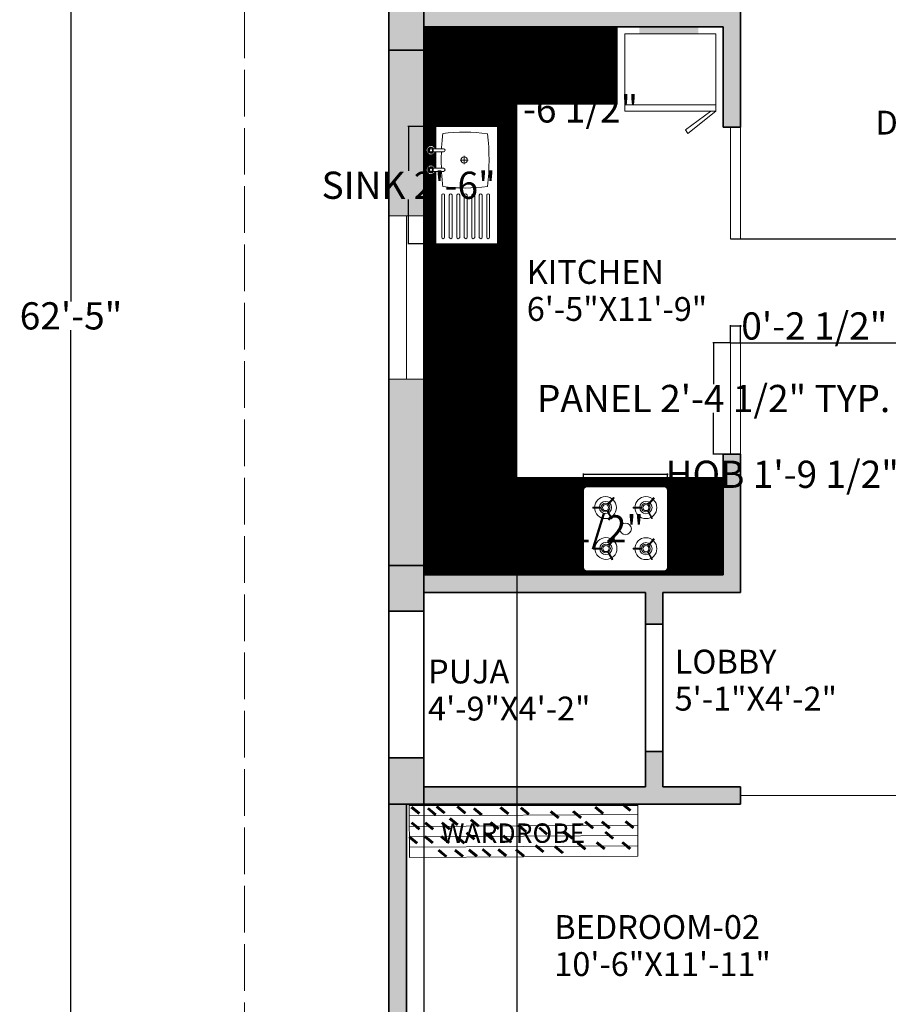
# Model space of a CAD drawing. Units: inches. Extents: x -17 to 892, y -721 to 172.
# Tile 2 of 11: x -12 to 212, y -462 to -209. Entities that reach past the tile are written whole.
import ezdxf

# ---------------------------------------------------------------- set-up
doc = ezdxf.new("R2010")
doc.units = ezdxf.units.IN
doc.header["$MEASUREMENT"] = 0
doc.linetypes.add('ACAD_ISO02W100', pattern=[15, 12, -3])
doc.layers.get('0').update_dxf_attribs({"color": 14})
for name, color, linetype, lineweight in [('A-ANNO-DIMS', 2, 'Continuous', 18), ('A-ANNO-TEXT', 7, 'Continuous', 18), ('A-AREA-IDEN', 7, 'Continuous', 18), ('A-COLS', 252, 'Continuous', 35), ('A-EQPM', 8, 'Continuous', 18), ('A-FLOR-CASE', 252, 'Continuous', 18), ('A-FLOR-FIXT', 8, 'Continuous', 18), ('A-FURN-PATT', 252, 'Continuous', 9), ('A-WALL-PATT', 14, 'Continuous', 13), ('C-PROP', 8, 'ACAD_ISO02W100', 18), ('doors', 4, 'Continuous', 18), ('furniture', 252, 'Continuous', 18), ('walls', 252, 'Continuous', 35), ('windows', 161, 'Continuous', 18)]:
    doc.layers.add(name, color=color, linetype=linetype, lineweight=lineweight)
doc.layers.add('A-COLS-PATT', color=254, linetype='Continuous', lineweight=13, true_color=0xd7ebd2)
doc.layers.add('A-FLOR-CASE-PATT', color=51, linetype='Continuous', lineweight=13, true_color=0xf8f6b0)
doc.styles.get("Standard").update_dxf_attribs({"font": 'arial.ttf'})
doc.dimstyles.get("Standard").update_dxf_attribs({"dimtxt": 7, "dimasz": 0.18, "dimexe": 0.18, "dimexo": 0.0625, "dimgap": 0.09, "dimtad": 0, "dimtih": 1, "dimtoh": 1, "dimzin": 0, "dimdsep": 46, "dimlunit": 3, "dimtxsty": 'Standard', "dimcen": 0.09, "dimadec": 0, "dimazin": 0, "dimtfac": 1, "dimtofl": 0, "dimtmove": 0, "dimatfit": 3, "dimfxl": 1, "dimtolj": 1, "dimtzin": 0, "dimarcsym": 0})

# ---------------------------------------------------------------- blocks, each defined once
blk = doc.blocks.new('A$C799204C7')
for p, q in [((0, 34.2), (17.99, 34.2)), ((0, 0), (0, 34.2)), ((2.32, 20.01), (2.32, 32.27)), ((3.13, 20.01), (3.13, 32.27)), ((4.48, 20.01), (4.48, 32.27)), ((5.29, 20.01), (5.29, 32.27)), ((6.64, 20.01), (6.64, 32.27)), ((7.45, 20.01), (7.45, 32.27)), ((8.85, 20.01), (8.85, 32.27)), ((9.66, 20.01), (9.66, 32.27)), ((11.01, 20.01), (11.01, 32.27)), ((11.82, 20.01), (11.82, 32.27)), ((13.22, 20.01), (13.22, 32.27)), ((14.03, 20.01), (14.03, 32.27)), ((15.42, 20.01), (15.42, 32.27)), ((16.24, 20.01), (16.24, 32.27)), ((17.99, 13.08), (17.99, 34.2)), ((18.59, 13.08), (15.71, 13.08)), ((15.71, 12.17), (18.59, 12.17)), ((17.99, 7.36), (17.99, 12.17)), ((8.52, 9.77), (10.9, 9.77)), ((9.73, 11), (9.73, 8.54)), ((18.59, 7.36), (15.71, 7.36)), ((15.71, 6.45), (18.59, 6.45)), ((17.99, 0), (17.99, 6.45)), ((0, 0), (17.99, 0))]:
    blk.add_line(p, q)
for centre, radius in [((19.38, 12.62), 0.684), ((19.38, 12.62), 0.456), ((9.7, 9.77), 0.916), ((19.38, 6.91), 0.684), ((19.38, 6.91), 0.456)]:
    blk.add_circle(centre, radius)
for centre, radius, start, end in [((2.72, 32.27), 0.407, 0, 180), ((4.88, 32.27), 0.407, 0, 180), ((7.05, 32.27), 0.407, 0, 180), ((9.25, 32.27), 0.407, 0, 180), ((11.42, 32.27), 0.407, 0, 180), ((13.62, 32.27), 0.407, 0, 180), ((15.83, 32.27), 0.407, 0, 180), ((2.72, 20.01), 0.407, 180, 0), ((67.33, 9.77), 64.88, 173.1952, 186.8048), ((9.53, -30.19), 48.1, 82.3437, 97.8966), ((4.88, 20.01), 0.407, 180, 0), ((7.05, 20.01), 0.407, 180, 0), ((9.25, 20.01), 0.407, 180, 0), ((11.42, 20.01), 0.407, 180, 0), ((13.62, 20.01), 0.407, 180, 0), ((15.83, 20.01), 0.407, 180, 0), ((-48.51, 9.77), 64.88, 2.9208, 6.8048), ((15.71, 12.62), 0.456, 90, 270), ((-48.51, 9.77), 64.88, 357.8723, 2.115), ((19.38, 12.62), 1.37, 199.6514, 160.3603), ((19.38, 12.62), 0.911, 210.3431, 149.7554), ((15.71, 6.91), 0.456, 90, 270), ((-48.51, 9.77), 64.88, 353.1952, 357.0665), ((19.38, 6.91), 1.37, 199.6514, 160.3603), ((19.38, 6.91), 0.911, 210.3431, 149.7554), ((9.53, 49.73), 48.1, 262.1034, 277.6563)]:
    blk.add_arc(centre, radius, start, end)
blk = doc.blocks.new('sink')
at = {"layer": 'furniture'}
for p, q in [((8718164203.894819, -1433730582.369047), (8718164201.504578, -1433730582.369047)), ((8718164202.684322, -1433730581.131674), (8718164202.684322, -1433730583.598095)), ((8718164196.150837, -1433730592.638258), (8718164196.150837, -1433730604.938997)), ((8718164196.967728, -1433730592.638258), (8718164196.967728, -1433730604.938997)), ((8718164198.365185, -1433730592.638258), (8718164198.365185, -1433730604.938997)), ((8718164199.182076, -1433730592.638258), (8718164199.182076, -1433730604.938997)), ((8718164200.579533, -1433730592.638258), (8718164200.579533, -1433730604.938997)), ((8718164201.396423, -1433730592.638258), (8718164201.396423, -1433730604.938997)), ((8718164202.748692, -1433730592.638258), (8718164202.748692, -1433730604.938997)), ((8718164203.565582, -1433730592.638258), (8718164203.565582, -1433730604.938997)), ((8718164204.963041, -1433730592.638258), (8718164204.963041, -1433730604.938997)), ((8718164205.779934, -1433730592.638258), (8718164205.779934, -1433730604.938997)), ((8718164207.1322, -1433730592.638258), (8718164207.1322, -1433730604.938997)), ((8718164207.949093, -1433730592.638258), (8718164207.949093, -1433730604.938997)), ((8718164209.301359, -1433730592.638258), (8718164209.301359, -1433730604.938997)), ((8718164210.118252, -1433730592.638258), (8718164210.118252, -1433730604.938997))]:
    blk.add_line(p, q, dxfattribs=at)
for centre, radius in [((8718164192.998869, -1433730579.495552), 0.685789), ((8718164192.998869, -1433730579.495552), 0.457192), ((8718164202.715019, -1433730582.369047), 0.919003), ((8718164192.998869, -1433730585.228166), 0.68579), ((8718164192.998869, -1433730585.228166), 0.68579), ((8718164192.998869, -1433730585.228166), 0.457192)]:
    blk.add_circle(centre, radius, dxfattribs=at)
for centre, radius, start, end in [((8718164196.559284, -1433730592.638258), 0.41045, 354.3355999, 185.6644001), ((8718164198.77363, -1433730592.638258), 0.41045, 354.3355999, 185.6644001), ((8718164200.98798, -1433730592.638258), 0.41045, 354.3355999, 185.6644001), ((8718164203.157139, -1433730592.638258), 0.41045, 354.3355999, 185.6644001), ((8718164205.371487, -1433730592.638258), 0.41045, 354.3355999, 185.6644001), ((8718164207.540646, -1433730592.640262), 0.41045, 354.3355999, 185.6644001), ((8718164209.709805, -1433730592.640262), 0.41045, 354.3355999, 185.6644001), ((8718164196.559284, -1433730604.938997), 0.408445, 180, 0), ((8718164198.77363, -1433730604.938997), 0.408445, 180, 0), ((8718164200.98798, -1433730604.938997), 0.408445, 180, 0), ((8718164203.157139, -1433730604.938997), 0.408445, 180, 0), ((8718164205.371487, -1433730604.938997), 0.408445, 180, 0), ((8718164207.540646, -1433730604.938997), 0.408445, 180, 0), ((8718164209.709805, -1433730604.938997), 0.408445, 180, 0)]:
    blk.add_arc(centre, radius, start, end, dxfattribs=at)
at = {"layer": 'furniture', "xscale": 1.0032, "yscale": 1.0032, "zscale": 1.0032, "rotation": 180}
blk.add_blockref('A$C799204C7', (8718164212.441259, -1433730572.566334), dxfattribs=at)
blk = doc.blocks.new('washbasin')
at = {"layer": 'furniture'}
blk.add_blockref('sink', (-8718164214.119328, 1433730589.721069), dxfattribs=at)
blk = doc.blocks.new('4bstove')
at = {"layer": 'furniture'}
for p, q in [((1452.73, 1446.21), (1452.73, 1448.61)), ((1452.98, 1446.22), (1452.98, 1448.61)), ((1464.44, 1446.34), (1464.44, 1448.73)), ((1464.69, 1446.34), (1464.69, 1448.73)), ((1451.74, 1444.45), (1449.67, 1443.25)), ((1451.87, 1444.23), (1449.79, 1443.04)), ((1453.91, 1444.27), (1455.74, 1442.73)), ((1463.45, 1444.58), (1461.38, 1443.38)), ((1463.57, 1444.36), (1461.5, 1443.17)), ((1465.46, 1444.21), (1467.29, 1442.67)), ((1465.62, 1444.4), (1467.45, 1442.86)), ((1453.75, 1444.08), (1455.58, 1442.54)), ((1452.69, 1434.81), (1452.69, 1437.2)), ((1452.94, 1434.81), (1452.94, 1437.2)), ((1464.44, 1434.81), (1464.44, 1437.2)), ((1464.69, 1434.81), (1464.69, 1437.2)), ((1451.7, 1433.04), (1449.63, 1431.85)), ((1463.45, 1433.04), (1461.38, 1431.85)), ((1451.82, 1432.83), (1449.75, 1431.63)), ((1453.71, 1432.67), (1455.54, 1431.13)), ((1453.87, 1432.86), (1455.7, 1431.33)), ((1463.57, 1432.83), (1461.5, 1431.63)), ((1465.46, 1432.67), (1467.29, 1431.13)), ((1465.62, 1432.86), (1467.45, 1431.33))]:
    blk.add_line(p, q, dxfattribs=at)
for points in [[(1447.5, 1427.38), (1469.5, 1427.38, 0.414214), (1470.5, 1428.38), (1470.5, 1450.38, 0.414214), (1469.5, 1451.38), (1447.5, 1451.38, 0.414214), (1446.5, 1450.38), (1446.5, 1428.38, 0.414214)], [(1453.75, 1444.97, 1), (1452, 1444.97, 1)], [(1465.46, 1445.1, 1), (1463.71, 1445.1, 1)], [(1453.71, 1433.56, 1), (1451.96, 1433.56, 1)], [(1465.46, 1433.56, 1), (1463.71, 1433.56, 1)]]:
    blk.add_lwpolyline(points, format="xyb", close=True, dxfattribs=at)
for points in [[(1454.12, 1444.97, 1), (1451.62, 1444.97, 1), (1454.12, 1444.97, 1)], [(1465.83, 1445.1, 1), (1463.33, 1445.1, 1), (1465.83, 1445.1, 1)], [(1454.08, 1433.56, 1), (1451.58, 1433.56, 1), (1454.08, 1433.56, 1)], [(1465.83, 1433.56, 1), (1463.33, 1433.56, 1), (1465.83, 1433.56, 1)]]:
    blk.add_lwpolyline(points, format="xyb", dxfattribs=at)
for centre, radius in [((1452.87, 1444.97), 3.14), ((1464.58, 1445.1), 3.14), ((1452.87, 1444.97), 1.75), ((1464.58, 1445.1), 1.75), ((1458.5, 1439.38), 1.67), ((1452.83, 1433.56), 3.14), ((1464.58, 1433.56), 3.14), ((1452.83, 1433.56), 1.75), ((1464.58, 1433.56), 1.75)]:
    blk.add_circle(centre, radius, dxfattribs=at)
for centre, start, end in [((1452.87, 1444.97), 88.2645, 92.2039), ((1464.58, 1445.1), 88.2645, 92.2039), ((1452.87, 1444.97), 208.188, 212.1274), ((1452.87, 1444.97), 318.1018, 322.0412), ((1464.58, 1445.1), 208.188, 212.1274), ((1464.58, 1445.1), 318.1018, 322.0412), ((1452.83, 1433.56), 88.2645, 92.2039), ((1464.58, 1433.56), 88.2645, 92.2039)]:
    blk.add_arc(centre, 3.64, start, end, dxfattribs=at)
blk = doc.blocks.new('stove')
at = {"layer": 'furniture', "xscale": 0.9, "yscale": 0.9, "zscale": 0.9, "rotation": 89.99999999999999}
blk.add_blockref('4bstove', (1295.44, -1312.65), dxfattribs=at)
blk = doc.blocks.new('WIN-42-FRAMED')
for p, q in [((0, 41.96), (9, 41.96)), ((0, 0), (0, 41.96)), ((0, 41.96), (4.5, 41.96)), ((4.5, 41.96), (4.5, 0)), ((9, 41.96), (9, 0)), ((9, 0), (0, 0))]:
    blk.add_line(p, q)
blk = doc.blocks.new('WARDROBE-59-PLAN')
for p, q in [((0, 13.37), (58.88, 13.37)), ((0.05, 13.37), (0.13, 0)), ((58.95, 0.34), (58.88, 13.71)), ((0.02, 10.69), (58.89, 11.04)), ((0.03, 8.02), (58.91, 8.36)), ((0.05, 5.35), (58.92, 5.69)), ((0.06, 2.67), (58.94, 3.02)), ((0.08, 0), (58.95, 0.34))]:
    blk.add_line(p, q)
blk = doc.blocks.new('DOOR-KITCHEN-PANEL')
for p, q in [((2.65, 28.72), (0, 28.72)), ((0, 28.72), (0, 0)), ((2.65, 0), (2.65, 28.72))]:
    blk.add_line(p, q)
blk = doc.blocks.new('*D50')
at = {"layer": 'A-ANNO-DIMS', "color": 0, "lineweight": -2, "transparency": 16777216}
for p, q in [((170.87, -291.63), (166.44, -291.63)), ((166.62, -291.81), (166.62, -302.28)), ((166.62, -320.17), (166.62, -309.7)), ((170.87, -320.35), (166.44, -320.35))]:
    blk.add_line(p, q, dxfattribs=at)
at = {"layer": 'A-ANNO-DIMS', "color": 0, "lineweight": 100, "transparency": 16777216}
for points in [[(166.59, -291.81), (166.65, -291.81), (166.62, -291.63)], [(166.59, -320.17), (166.65, -320.17), (166.62, -320.35)]]:
    blk.add_solid(points, dxfattribs=at)
at = {"layer": 'Defpoints', "color": 0, "lineweight": 100, "transparency": 16777216}
for p in [(166.62, -291.63), (170.93, -291.63), (170.93, -320.35)]:
    blk.add_point(p, dxfattribs=at)
at = {"layer": 'A-ANNO-DIMS', "color": 0, "transparency": 16777216, "insert": (166.62, -305.99), "char_height": 7, "attachment_point": 5}
blk.add_mtext('\\A1;PANEL 2\'-4 1/2" TYP.', dxfattribs=at)
blk = doc.blocks.new('*D51')
at = {"layer": 'A-ANNO-DIMS', "color": 0, "lineweight": -2, "transparency": 16777216}
for p, q in [((170.93, -291.56), (170.93, -287.14)), ((171.11, -287.32), (173.4, -287.32)), ((173.58, -291.56), (173.58, -287.14)), ((173.58, -287.32), (173.76, -287.32))]:
    blk.add_line(p, q, dxfattribs=at)
at = {"layer": 'A-ANNO-DIMS', "color": 0, "lineweight": 100, "transparency": 16777216}
for points in [[(171.11, -287.29), (171.11, -287.35), (170.93, -287.32)], [(173.4, -287.29), (173.4, -287.35), (173.58, -287.32)]]:
    blk.add_solid(points, dxfattribs=at)
at = {"layer": 'Defpoints', "color": 0, "lineweight": 100, "transparency": 16777216}
for p in [(173.58, -287.32), (170.93, -291.63), (173.58, -291.63)]:
    blk.add_point(p, dxfattribs=at)
at = {"layer": 'A-ANNO-DIMS', "color": 0, "transparency": 16777216, "insert": (203.34, -287.32), "char_height": 7, "attachment_point": 5}
blk.add_mtext('\\A1;0\'-2 1/2" TYP.', dxfattribs=at)
blk = doc.blocks.new('*D52')
at = {"layer": 'A-ANNO-DIMS', "color": 0, "lineweight": -2, "transparency": 16777216}
for p, q in [((92.63, -236), (87.98, -236)), ((88.16, -236.18), (88.16, -247.4)), ((88.16, -266.04), (88.16, -254.82)), ((92.63, -266.22), (87.98, -266.22))]:
    blk.add_line(p, q, dxfattribs=at)
at = {"layer": 'A-ANNO-DIMS', "color": 0, "lineweight": 100, "transparency": 16777216}
for points in [[(88.13, -236.18), (88.19, -236.18), (88.16, -236)], [(88.13, -266.04), (88.19, -266.04), (88.16, -266.22)]]:
    blk.add_solid(points, dxfattribs=at)
at = {"layer": 'Defpoints', "color": 0, "lineweight": 100, "transparency": 16777216}
for p in [(88.16, -236), (92.69, -236), (92.69, -266.22)]:
    blk.add_point(p, dxfattribs=at)
at = {"layer": 'A-ANNO-DIMS', "color": 0, "transparency": 16777216, "insert": (88.16, -251.11), "char_height": 7, "attachment_point": 5}
blk.add_mtext('\\A1;SINK 2\'-6"', dxfattribs=at)
blk = doc.blocks.new('*D53')
at = {"layer": 'A-ANNO-DIMS', "color": 0, "lineweight": -2, "transparency": 16777216}
for p, q in [((92.69, -235.94), (92.69, -231.29)), ((92.87, -231.47), (110.84, -231.47)), ((111.02, -235.94), (111.02, -231.29)), ((111.02, -231.47), (111.2, -231.47))]:
    blk.add_line(p, q, dxfattribs=at)
at = {"layer": 'A-ANNO-DIMS', "color": 0, "lineweight": 100, "transparency": 16777216}
for points in [[(92.87, -231.44), (92.87, -231.5), (92.69, -231.47)], [(110.84, -231.44), (110.84, -231.5), (111.02, -231.47)]]:
    blk.add_solid(points, dxfattribs=at)
at = {"layer": 'Defpoints', "color": 0, "lineweight": 100, "transparency": 16777216}
for p in [(111.02, -231.47), (92.69, -236), (111.02, -236)]:
    blk.add_point(p, dxfattribs=at)
at = {"layer": 'A-ANNO-DIMS', "color": 0, "transparency": 16777216, "insert": (128.42, -231.47), "char_height": 7, "attachment_point": 5}
blk.add_mtext('\\A1;1\'-6 1/2"', dxfattribs=at)
blk = doc.blocks.new('*D54')
at = {"layer": 'A-ANNO-DIMS', "color": 0, "lineweight": -2, "transparency": 16777216}
for p, q in [((133.16, -328.67), (133.16, -325.31)), ((133.34, -325.49), (154.58, -325.49)), ((154.76, -328.67), (154.76, -325.31)), ((154.76, -325.49), (154.94, -325.49))]:
    blk.add_line(p, q, dxfattribs=at)
at = {"layer": 'A-ANNO-DIMS', "color": 0, "lineweight": 100, "transparency": 16777216}
for points in [[(133.34, -325.46), (133.34, -325.52), (133.16, -325.49)], [(154.58, -325.46), (154.58, -325.52), (154.76, -325.49)]]:
    blk.add_solid(points, dxfattribs=at)
at = {"layer": 'Defpoints', "color": 0, "lineweight": 100, "transparency": 16777216}
for p in [(154.76, -325.49), (133.16, -328.73), (154.76, -328.73)]:
    blk.add_point(p, dxfattribs=at)
at = {"layer": 'A-ANNO-DIMS', "color": 0, "transparency": 16777216, "insert": (184.26, -325.49), "char_height": 7, "attachment_point": 5}
blk.add_mtext('\\A1;HOB 1\'-9 1/2"', dxfattribs=at)
blk = doc.blocks.new('*D55')
at = {"layer": 'A-ANNO-DIMS', "color": 0, "lineweight": -2, "transparency": 16777216}
for p, q in [((133.1, -328.73), (129.74, -328.73)), ((129.92, -328.91), (129.92, -335.82)), ((129.92, -350.15), (129.92, -343.24)), ((133.1, -350.33), (129.74, -350.33))]:
    blk.add_line(p, q, dxfattribs=at)
at = {"layer": 'A-ANNO-DIMS', "color": 0, "lineweight": 100, "transparency": 16777216}
for points in [[(129.89, -328.91), (129.95, -328.91), (129.92, -328.73)], [(129.89, -350.15), (129.95, -350.15), (129.92, -350.33)]]:
    blk.add_solid(points, dxfattribs=at)
at = {"layer": 'Defpoints', "color": 0, "lineweight": 100, "transparency": 16777216}
for p in [(129.92, -328.73), (133.16, -328.73), (133.16, -350.33)]:
    blk.add_point(p, dxfattribs=at)
at = {"layer": 'A-ANNO-DIMS', "color": 0, "transparency": 16777216, "insert": (129.92, -339.53), "char_height": 7, "attachment_point": 5}
blk.add_mtext('\\A1;1\'-9 1/2"', dxfattribs=at)
blk = doc.blocks.new('*D57')
at = {"layer": 'A-ANNO-DIMS', "color": 0, "lineweight": -2, "transparency": 16777216}
for p, q in [((83.02, 89.9), (1.11, 89.9)), ((1.29, 89.72), (1.29, -281.05)), ((1.29, -659.16), (1.29, -288.38)), ((83.02, -659.34), (1.11, -659.34))]:
    blk.add_line(p, q, dxfattribs=at)
at = {"layer": 'A-ANNO-DIMS', "color": 0, "lineweight": 100, "transparency": 16777216}
for points in [[(1.26, 89.72), (1.32, 89.72), (1.29, 89.9)], [(1.26, -659.16), (1.32, -659.16), (1.29, -659.34)]]:
    blk.add_solid(points, dxfattribs=at)
at = {"layer": 'Defpoints', "color": 0, "lineweight": 100, "transparency": 16777216}
for p in [(1.29, 89.9), (83.08, 89.9), (83.08, -659.34)]:
    blk.add_point(p, dxfattribs=at)
at = {"layer": 'A-ANNO-DIMS', "color": 0, "transparency": 16777216, "insert": (1.29, -284.72), "char_height": 7, "attachment_point": 5}
blk.add_mtext('\\A1;62\'-5"', dxfattribs=at)
blk = doc.blocks.new('*D60')
at = {"layer": 'A-ANNO-DIMS', "color": 0, "lineweight": -2, "transparency": 16777216}
for p, q in [((116.03, -326.38), (116.03, -704.12)), ((92.08, -351.45), (92.08, -704.12)), ((92.26, -703.94), (94.6, -703.94)), ((115.85, -703.94), (113.51, -703.94))]:
    blk.add_line(p, q, dxfattribs=at)
at = {"layer": 'A-ANNO-DIMS', "color": 0, "lineweight": 100, "transparency": 16777216}
for points in [[(92.26, -703.91), (92.26, -703.97), (92.08, -703.94)], [(115.85, -703.91), (115.85, -703.97), (116.03, -703.94)]]:
    blk.add_solid(points, dxfattribs=at)
at = {"layer": 'Defpoints', "color": 0, "lineweight": 100, "transparency": 16777216}
for p in [(116.03, -326.32), (92.08, -351.39), (116.03, -703.94)]:
    blk.add_point(p, dxfattribs=at)
at = {"layer": 'A-ANNO-DIMS', "color": 0, "transparency": 16777216, "insert": (104.05, -703.94), "char_height": 7, "attachment_point": 5}
blk.add_mtext('\\A1;2\'-0"', dxfattribs=at)
blk = doc.blocks.new('*D61')
at = {"layer": 'A-ANNO-DIMS', "color": 0, "lineweight": -2, "transparency": 16777216}
for p, q in [((170.99, -264.92), (841.36, -264.92)), ((841.18, -265.1), (841.18, -274.56)), ((841.18, -291.45), (841.18, -281.98)), ((170.99, -291.63), (841.36, -291.63))]:
    blk.add_line(p, q, dxfattribs=at)
at = {"layer": 'A-ANNO-DIMS', "color": 0, "lineweight": 100, "transparency": 16777216}
for points in [[(841.15, -265.1), (841.21, -265.1), (841.18, -264.92)], [(841.15, -291.45), (841.21, -291.45), (841.18, -291.63)]]:
    blk.add_solid(points, dxfattribs=at)
at = {"layer": 'Defpoints', "color": 0, "lineweight": 100, "transparency": 16777216}
for p in [(170.93, -264.92), (170.93, -291.63), (841.18, -291.63)]:
    blk.add_point(p, dxfattribs=at)
at = {"layer": 'A-ANNO-DIMS', "color": 0, "transparency": 16777216, "insert": (841.18, -278.27), "char_height": 7, "attachment_point": 5}
blk.add_mtext('\\A1;2\'-2 1/2"', dxfattribs=at)

msp = doc.modelspace()

# ---------------------------------------------------------------- hatches: boundary and pattern name
at = {"layer": 'A-COLS-PATT'}
h = msp.add_hatch(color=256, dxfattribs=at)
h.dxf.hatch_style = 1
h.paths.add_polyline_path([(92.084, 61.611), (83.084, 61.611), (83.084, 43.692), (92.084, 43.692)])
h.paths.add_polyline_path([(347.084, 61.611), (338.084, 61.611), (338.084, 43.692), (347.084, 43.692)])
h.paths.add_polyline_path([(222.053, 61.611), (209.95, 61.611), (209.95, 52.611), (222.053, 52.611)])
h.paths.add_polyline_path([(284.798, 61.611), (274.584, 61.611), (274.584, 52.611), (284.798, 52.611)])
h.paths.add_polyline_path([(223.084, -106.389), (214.084, -106.389), (214.084, -119.959), (223.084, -119.959)])
h.paths.add_polyline_path([(347.084, -148.653), (338.084, -148.653), (338.084, -172.24), (347.084, -172.24)])
h.paths.add_polyline_path([(92.084, -102.402), (83.084, -102.402), (83.084, -119.959), (92.084, -119.959)])
h.paths.add_polyline_path([(92.084, -205.889), (83.084, -205.889), (83.084, -216.319), (92.084, -216.319)])
h.paths.add_polyline_path([(347.084, -349.073), (338.084, -349.073), (338.084, -372.66), (347.084, -372.66)])
h.paths.add_polyline_path([(347.084, -610.134), (338.084, -610.134), (338.084, -614.389), (338.084, -623.342), (347.084, -623.342)])
h.paths.add_polyline_path([(221.166, -610.357), (214.084, -610.357), (214.084, -623.389), (219.084, -623.389), (221.166, -623.389), (221.166, -621.723)])
h.paths.add_polyline_path([(90.166, -610.357), (83.084, -610.357), (83.084, -623.389), (90.166, -623.389)])
h.paths.add_polyline_path([(223.084, -401.64), (214.084, -401.64), (214.084, -410.389), (223.084, -410.389)])
h.paths.add_polyline_path([(223.084, -356.889), (214.084, -356.889), (214.084, -369.273), (223.084, -369.273)])
h.paths.add_polyline_path([(92.084, -398.492), (83.084, -398.492), (83.084, -410.389), (92.084, -410.389)])
h.paths.add_polyline_path([(92.084, -348.918), (83.084, -348.918), (83.084, -360.706), (92.084, -360.706)])
at = {"layer": 'A-EQPM'}
h = msp.add_hatch(color=256, dxfattribs=at)
h.dxf.hatch_style = 1
h.paths.add_polyline_path([(147.501, -210.552), (147.501, -212.116), (162.733, -212.116), (162.733, -210.552)])
at = {"layer": 'A-FLOR-CASE-PATT'}
h = msp.add_hatch(dxfattribs=at)
h.set_pattern_fill('ANSI31', color=256)
h.paths.add_polyline_path([(116.026, -230.269), (141.791, -230.269), (141.791, -210.389), (92.084, -210.389), (92.084, -351.389), (169.084, -351.389), (169.084, -326.317), (116.026, -326.317)])
h.paths.add_polyline_path([(134.062, -328.728), (153.862, -328.728, -0.4142136), (154.762, -329.628), (154.762, -349.428, -0.4142136), (153.862, -350.328), (134.062, -350.328, -0.4142136), (133.162, -349.428), (133.162, -329.628, -0.4142136)], flags=16)
h.paths.add_polyline_path([(140.538, -331.822), (140.828, -331.477, -0.0171906), (141, -331.621), (140.711, -331.966, -0.2116406), (141.637, -334.057, -0.2564461), (140.33, -336.439), (140.555, -336.829, -0.0171907), (140.36, -336.942), (140.135, -336.552, -0.5505708), (135.994, -334.183), (135.544, -334.183, -0.0171907), (135.543, -333.958), (135.993, -333.958, -0.6105283)], flags=0)
h.paths.add_polyline_path([(95.123, -266.222), (95.123, -247.559), (95.035, -247.559, -5.8284271), (95.035, -246.754), (95.123, -246.754), (95.123, -242.51), (95.035, -242.51, -5.8284271), (95.035, -241.705), (95.123, -241.705), (95.123, -236.004), (111.02, -236.004), (111.02, -266.222)], flags=16)
h.paths.add_polyline_path([(140.389, -334.057, -1), (137.239, -334.057, -1)], flags=0)
h.paths.add_polyline_path([(138.814, -332.932, -1), (138.814, -335.182, -1)], flags=0)
h.paths.add_polyline_path([(102.483, -264.516), (102.483, -253.683, -1), (103.203, -253.683), (103.203, -264.516, -1)], flags=0)
h.paths.add_polyline_path([(102.483, -264.516), (102.483, -253.718, -0.9999734), (103.203, -253.647), (103.203, -264.516, -1)], flags=0)
h.paths.add_polyline_path([(104.434, -264.517), (104.434, -253.683), (104.434, -253.683), (104.434, -253.718, -0.9999873), (105.153, -253.647), (105.153, -264.516, -0.9990341)], flags=0)
h.paths.add_polyline_path([(100.573, -264.516), (100.573, -253.683, -1), (101.292, -253.683), (101.292, -264.516, -1)], flags=0)
h.paths.add_polyline_path([(100.573, -264.516), (100.573, -253.718, -0.9999867), (101.292, -253.647), (101.292, -264.516, -1)], flags=0)
h.paths.add_polyline_path([(107.063, -253.649), (107.063, -264.516), (107.063, -264.516), (107.063, -264.516, -1), (106.344, -264.516), (106.344, -264.516, 1.0006251), (107.063, -264.516), (107.063, -253.682, 0.9998404), (106.344, -253.683), (106.344, -253.72, -1)], flags=0)
h.paths.add_polyline_path([(99.342, -264.516), (99.342, -264.516), (99.342, -264.516, -1), (98.623, -264.516), (98.623, -264.516, 1.0009121), (99.342, -264.516), (99.342, -253.682, 0.9990888), (98.623, -253.683), (98.623, -253.718, -1.0000023), (99.342, -253.647)], flags=0)
h.paths.add_polyline_path([(138.814, -333.27, -1), (138.814, -334.845, -1)], flags=0)
h.paths.add_polyline_path([(108.254, -264.517), (108.254, -253.683), (108.254, -253.683), (108.254, -253.72, -0.9999895), (108.974, -253.649), (108.974, -264.516, -0.9990924)], flags=0)
h.paths.add_polyline_path([(96.672, -264.517), (96.672, -253.683), (96.672, -253.683), (96.672, -253.718, -0.9999761), (97.392, -253.647), (97.392, -264.516, -0.9987804)], flags=0)
h.paths.add_polyline_path([(140.653, -342.358), (140.942, -342.013, -0.0171906), (141.115, -342.157), (140.826, -342.502, -0.2116406), (141.752, -344.593, -0.2564461), (140.445, -346.975), (140.67, -347.365, -0.0171907), (140.475, -347.478), (140.25, -347.088, -0.5505708), (136.109, -344.719), (135.659, -344.719, -0.0171907), (135.658, -344.494), (136.108, -344.494, -0.6105283)], flags=0)
h.paths.add_polyline_path([(140.504, -344.593, -1), (137.354, -344.593, -1)], flags=0)
h.paths.add_polyline_path([(138.929, -343.468, -1), (138.929, -345.718, -1)], flags=0)
h.paths.add_polyline_path([(145.925, -333.958), (146.375, -333.958, -0.9825922), (152.02, -334.057, -0.9779445), (146.376, -334.183), (145.926, -334.183, -0.0171907)], flags=0)
h.paths.add_polyline_path([(145.465, -339.528, -1), (142.458, -339.528, -1)], flags=0)
h.paths.add_polyline_path([(138.929, -343.806, -1), (138.929, -345.381, -1)], flags=0)
h.paths.add_polyline_path([(150.771, -334.057, -1), (147.621, -334.057, -1)], flags=0)
h.paths.add_polyline_path([(149.196, -332.932, -1), (149.196, -335.182, -1)], flags=0)
h.paths.add_polyline_path([(149.196, -333.27, -1), (149.196, -334.845, -1)], flags=0)
h.paths.add_polyline_path([(152.02, -344.632, -0.9779445), (146.376, -344.758), (145.926, -344.758, -0.0171907), (145.925, -344.533), (146.375, -344.533, -0.9825922)], flags=0)
h.paths.add_polyline_path([(150.771, -344.632, -1), (147.621, -344.632, -1)], flags=0)
h.paths.add_polyline_path([(149.196, -343.507, -1), (149.196, -345.757, -1)], flags=0)
h.paths.add_polyline_path([(149.196, -343.844, -1), (149.196, -345.419, -1)], flags=0)
h.paths.add_polyline_path([(93.494, -247.156, -1), (94.299, -247.156, -1)], flags=0)
h.paths.add_polyline_path([(102.427, -245.721), (102.427, -245.447, -0.4044618), (101.644, -244.638), (101.644, -244.638, 0.4044617), (102.427, -245.447), (102.427, -244.638), (101.644, -244.638, 0.4044618), (102.427, -245.447), (102.427, -245.447, -0.4044619), (101.644, -244.638), (101.388, -244.638), (101.388, -244.638), (101.644, -244.638, -0.404462), (102.427, -243.829), (102.427, -243.548), (102.427, -243.548), (102.427, -243.829, -0.4240328), (103.263, -244.638), (103.263, -244.638, 0.4240327), (102.427, -243.829), (102.427, -244.638), (103.263, -244.638, 0.4240328), (102.427, -243.829), (102.427, -243.829, -0.4240329), (103.263, -244.638), (103.493, -244.638), (103.493, -244.638), (103.263, -244.638, -0.424033), (102.427, -245.447), (102.427, -245.721)], flags=0)
h.paths.add_polyline_path([(93.494, -242.107, -1), (94.299, -242.107, -1)], flags=0)
at = {"layer": 'A-FURN-PATT'}
h = msp.add_hatch(dxfattribs=at)
h.set_pattern_fill('ANSI31', color=256, scale=0.8475126, angle=95.46701, style=0)
h.paths.add_polyline_path([(88.161, -419.012), (90.158, -420.66), (90.495, -420.252), (88.498, -418.604)])
h.paths.add_polyline_path([(95.711, -422.414), (97.708, -424.062), (98.045, -423.654), (96.048, -422.006)], flags=0)
h.paths.add_polyline_path([(92.222, -418.861), (94.219, -420.509), (94.556, -420.1), (92.559, -418.452)], flags=0)
h.paths.add_polyline_path([(88.733, -415.37), (90.73, -417.018), (91.067, -416.609), (89.07, -414.961)], flags=0)
h.paths.add_polyline_path([(99.976, -422.359), (101.973, -424.007), (102.31, -423.599), (100.313, -421.951)], flags=0)
h.paths.add_polyline_path([(96.366, -418.91), (98.363, -420.558), (98.7, -420.149), (96.704, -418.501)], flags=0)
h.paths.add_polyline_path([(92.307, -415.349), (94.304, -416.997), (94.641, -416.588), (92.645, -414.94)], flags=0)
h.paths.add_polyline_path([(88.735, -411.32), (90.732, -412.968), (91.069, -412.559), (89.072, -410.911)], flags=0)
h.paths.add_polyline_path([(103.536, -422.338), (105.533, -423.986), (105.87, -423.577), (103.873, -421.929)], flags=0)
h.paths.add_polyline_path([(100.294, -419.009), (102.291, -420.657), (102.628, -420.248), (100.631, -418.6)], flags=0)
h.paths.add_polyline_path([(96.601, -415.324), (98.598, -416.972), (98.935, -416.563), (96.939, -414.915)], flags=0)
h.paths.add_polyline_path([(92.978, -411.618), (94.975, -413.266), (95.312, -412.858), (93.315, -411.21)], flags=0)
h.paths.add_polyline_path([(107.045, -422.192), (109.042, -423.841), (109.379, -423.432), (107.382, -421.784)], flags=0)
h.paths.add_polyline_path([(102.9, -417.96), (104.897, -419.608), (105.235, -419.2), (103.238, -417.551)], flags=0)
h.paths.add_polyline_path([(98.596, -414.24), (100.593, -415.888), (100.93, -415.479), (98.933, -413.831)], flags=0)
h.paths.add_polyline_path([(95.233, -411.197), (97.23, -412.845), (97.567, -412.437), (95.57, -410.789)], flags=0)
h.paths.add_polyline_path([(111.102, -422.204), (113.099, -423.853), (113.436, -423.444), (111.44, -421.796)], flags=0)
h.paths.add_polyline_path([(107.481, -417.933), (109.478, -419.581), (109.815, -419.173), (107.818, -417.525)], flags=0)
h.paths.add_polyline_path([(104.015, -414.593), (106.012, -416.241), (106.349, -415.833), (104.352, -414.185)], flags=0)
h.paths.add_polyline_path([(100.562, -411.218), (102.559, -412.866), (102.896, -412.458), (100.899, -410.809)], flags=0)
h.paths.add_polyline_path([(115.677, -422.257), (117.674, -423.905), (118.011, -423.496), (116.014, -421.848)], flags=0)
h.paths.add_polyline_path([(112.346, -418.758), (114.343, -420.406), (114.68, -419.997), (112.683, -418.349)], flags=0)
h.paths.add_polyline_path([(109.137, -415.25), (111.134, -416.898), (111.471, -416.49), (109.474, -414.842)], flags=0)
h.paths.add_polyline_path([(104.784, -411.725), (106.781, -413.373), (107.118, -412.964), (105.121, -411.316)], flags=0)
h.paths.add_polyline_path([(120.666, -421.245), (122.663, -422.894), (123, -422.485), (121.003, -420.837)], flags=0)
h.paths.add_polyline_path([(116.181, -416.035), (118.178, -417.683), (118.515, -417.275), (116.518, -415.627)], flags=0)
h.paths.add_polyline_path([(111.617, -411.439), (113.614, -413.087), (113.951, -412.679), (111.954, -411.031)], flags=0)
h.paths.add_polyline_path([(125.695, -421.461), (127.692, -423.11), (128.029, -422.701), (126.032, -421.053)], flags=0)
h.paths.add_polyline_path([(121.62, -416.617), (123.617, -418.265), (123.954, -417.857), (121.957, -416.209)], flags=0)
h.paths.add_polyline_path([(116.849, -411.531), (118.846, -413.179), (119.183, -412.771), (117.186, -411.123)], flags=0)
h.paths.add_polyline_path([(131.495, -420.466), (133.492, -422.114), (133.829, -421.705), (131.832, -420.057)], flags=0)
h.paths.add_polyline_path([(128.134, -417.812), (130.131, -419.46), (130.468, -419.052), (128.471, -417.404)], flags=0)
h.paths.add_polyline_path([(124.548, -412.487), (126.545, -414.135), (126.882, -413.726), (124.885, -412.078)], flags=0)
h.paths.add_polyline_path([(130.298, -412.453), (132.295, -414.101), (132.632, -413.692), (130.635, -412.044)], flags=0)
h.paths.add_polyline_path([(138.589, -417.751), (140.586, -419.399), (140.923, -418.99), (138.926, -417.342)], flags=0)
h.paths.add_polyline_path([(133.45, -415.108), (135.447, -416.756), (135.784, -416.347), (133.787, -414.699)], flags=0)
h.paths.add_polyline_path([(136.409, -420.437), (138.406, -422.085), (138.743, -421.676), (136.746, -420.028)], flags=0)
h.paths.add_polyline_path([(142.996, -420.398), (144.992, -422.046), (145.33, -421.638), (143.333, -419.99)], flags=0)
h.paths.add_polyline_path([(143.801, -415.047), (145.798, -416.695), (146.135, -416.287), (144.138, -414.639)], flags=0)
h.paths.add_polyline_path([(137.737, -415.083), (139.734, -416.731), (140.071, -416.322), (138.074, -414.674)], flags=0)
h.paths.add_polyline_path([(143.038, -410.598), (145.035, -412.246), (145.372, -411.837), (143.375, -410.189)], flags=0)
h.paths.add_polyline_path([(136.04, -411.322), (138.037, -412.97), (138.374, -412.562), (136.377, -410.913)], flags=0)
at = {"layer": 'A-WALL-PATT'}
h = msp.add_hatch(color=256, dxfattribs=at)
h.dxf.hatch_style = 1
h.paths.add_polyline_path([(111.26, 61.611), (92.084, 61.611), (92.084, 52.611), (111.26, 52.611)])
h.paths.add_polyline_path([(209.95, 61.611), (179.154, 61.611), (179.154, 52.611), (209.95, 52.611)])
h.paths.add_polyline_path([(338.084, 61.611), (284.798, 61.611), (284.798, 52.611), (338.084, 52.611)])
h.paths.add_polyline_path([(279.084, 23.861), (274.584, 23.861), (274.584, -0.389), (279.084, -0.389)])
h.paths.add_polyline_path([(279.084, 52.611), (274.584, 52.611), (274.584, 46.881), (276.834, 46.881), (279.084, 46.881)])
h.paths.add_polyline_path([(279.084, -0.389), (274.584, -0.389), (274.584, -4.889), (279.084, -4.889)])
h.paths.add_polyline_path([(304.22, -0.389), (279.084, -0.389), (279.084, -4.889), (304.22, -4.889)])
h.paths.add_polyline_path([(347.084, 43.692), (338.084, 43.692), (338.084, -148.653), (347.084, -148.653)])
h.paths.add_polyline_path([(338.084, -154.889), (264.103, -154.889), (264.103, -163.889), (338.084, -163.889)])
h.paths.add_polyline_path([(223.084, -119.959), (214.084, -119.959), (214.084, -163.889), (223.084, -163.889)])
h.paths.add_polyline_path([(218.584, 52.611), (214.084, 52.611), (214.084, -106.389), (218.584, -106.389)])
h.paths.add_polyline_path([(92.084, -8.943), (83.084, -8.943), (83.084, -49.69), (87.584, -49.69), (92.084, -49.69)])
h.paths.add_polyline_path([(92.084, 43.692), (83.084, 43.692), (83.084, 33.018), (87.584, 33.018), (92.084, 33.018)])
h.paths.add_polyline_path([(92.084, -91.651), (83.084, -91.651), (83.084, -102.402), (92.084, -102.402)])
h.paths.add_polyline_path([(92.084, -119.959), (83.084, -119.959), (83.084, -151.855), (87.584, -151.855), (92.084, -151.855)])
h.paths.add_polyline_path([(173.584, -108.639), (173.584, -106.389), (173.084, -106.389), (92.084, -106.389), (92.084, -110.889), (169.084, -110.889), (169.084, -176.029), (173.584, -176.029)])
h.paths.add_polyline_path([(92.084, -185.221), (83.084, -185.221), (83.084, -205.889), (92.084, -205.889)])
h.paths.add_polyline_path([(92.084, -216.319), (83.084, -216.319), (83.084, -259.015), (87.584, -259.015), (92.084, -259.015)])
h.paths.add_polyline_path([(173.584, -205.889), (92.084, -205.889), (92.084, -210.389), (169.084, -210.389), (169.084, -236.193), (173.584, -236.193)])
h.paths.add_polyline_path([(92.084, -300.976), (83.084, -300.976), (83.084, -348.918), (92.084, -348.918)])
h.paths.add_polyline_path([(87.584, -410.389), (83.084, -410.389), (83.084, -610.357), (87.584, -610.357)])
h.paths.add_polyline_path([(115.523, -614.389), (90.166, -614.389), (90.166, -623.389), (115.523, -623.389)])
h.paths.add_polyline_path([(214.084, -614.389), (174.149, -614.389), (174.149, -623.389), (214.084, -623.389)])
h.paths.add_polyline_path([(219.084, -410.389), (214.084, -410.389), (214.084, -610.357), (219.084, -610.357)])
h.paths.add_polyline_path([(347.084, -372.66), (338.084, -372.66), (338.084, -610.134), (347.084, -610.134)])
h.paths.add_polyline_path([(347.084, -172.24), (338.084, -172.24), (338.084, -349.073), (347.084, -349.073)])
h.paths.add_polyline_path([(338.084, -356.889), (317.618, -356.889), (317.618, -365.889), (338.084, -365.889)])
h.paths.add_polyline_path([(267.632, -356.889), (263.828, -356.889), (263.828, -365.889), (267.632, -365.889)])
h.paths.add_polyline_path([(223.084, -369.273), (214.084, -369.273), (214.084, -401.64), (223.084, -401.64)])
h = msp.add_hatch(color=256, dxfattribs=at)
h.dxf.hatch_style = 1
h.paths.add_polyline_path([(267.203, -620.057), (262.274, -620.057), (262.274, -623.389), (267.203, -623.389)])
h.paths.add_polyline_path([(338.084, -620.057), (335.531, -620.057), (335.531, -623.389), (338.084, -623.389)])
h.paths.add_polyline_path([(173.584, -405.889), (153.584, -405.889), (153.584, -396.835), (149.084, -396.835), (149.084, -405.889), (92.084, -405.889), (92.084, -410.389), (173.584, -410.389)])
h.paths.add_polyline_path([(153.584, -355.889), (173.584, -355.889), (173.584, -320.35), (169.084, -320.35), (169.084, -351.389), (92.084, -351.389), (92.084, -355.889), (149.084, -355.889), (149.084, -364.083), (153.584, -364.083)])

# ---------------------------------------------------------------- linework, layer by layer
at = {"layer": 'A-COLS'}
for p, q in [((83.084, -216.319), (92.084, -216.319)), ((83.084, -348.918), (92.084, -348.918)), ((83.084, -360.706), (92.084, -360.706)), ((83.084, -360.706), (92.084, -360.706)), ((83.084, -398.492), (92.084, -398.492)), ((83.084, -410.389), (92.084, -410.389))]:
    msp.add_line(p, q, dxfattribs=at)
at = {"layer": 'A-EQPM'}
for p, q in [((143.758, -232.042), (143.758, -212.116)), ((143.758, -212.116), (167.222, -212.116)), ((167.222, -212.116), (167.222, -232.042)), ((167.222, -230.447), (143.758, -230.447)), ((167.222, -232.042), (143.758, -232.042)), ((159.42, -236.843), (165.941, -232.042)), ((167.222, -232.042), (159.959, -237.756)), ((159.959, -237.756), (159.42, -236.843))]:
    msp.add_line(p, q, dxfattribs=at)
at = {"layer": 'A-FLOR-CASE'}
for p, q in [((141.791, -230.269), (141.791, -210.389)), ((116.026, -326.317), (116.026, -230.269)), ((116.026, -230.269), (141.791, -230.269)), ((169.084, -326.317), (116.026, -326.317)), ((113.852, -419.933), (113.852, -419.933))]:
    msp.add_line(p, q, dxfattribs=at)
at = {"layer": 'C-PROP'}
msp.add_line((45.892, -623.389), (45.892, 61.611), dxfattribs=at)
at = {"layer": 'doors'}
msp.add_line((173.584, -408.139), (214.084, -408.139), dxfattribs=at)
at = {"layer": 'walls'}
for p, q in [((83.084, -623.389), (83.084, 61.611)), ((92.084, -410.389), (92.084, 61.611)), ((173.584, -236.193), (173.584, -205.889)), ((92.084, -210.389), (169.084, -210.389)), ((169.084, -236.193), (169.084, -210.389)), ((169.084, -236.193), (173.584, -236.193)), ((169.084, -351.389), (169.084, -320.35)), ((169.084, -320.35), (173.584, -320.35)), ((173.584, -355.889), (173.584, -320.35)), ((92.084, -351.389), (169.084, -351.389)), ((92.084, -355.889), (149.084, -355.889)), ((149.084, -405.889), (149.084, -355.889)), ((153.584, -405.889), (153.584, -355.889)), ((153.584, -355.889), (173.584, -355.889)), ((149.084, -364.083), (153.584, -364.083)), ((149.084, -396.835), (153.584, -396.835)), ((92.084, -405.889), (149.084, -405.889)), ((153.584, -405.889), (173.584, -405.889)), ((173.584, -405.889), (173.584, -410.389)), ((87.584, -610.357), (87.584, -410.389)), ((92.084, -410.389), (173.584, -410.389))]:
    msp.add_line(p, q, dxfattribs=at)

# ---------------------------------------------------------------- block references
at = {"layer": 'A-EQPM'}
msp.add_blockref('stove', (143.962, -339.528), dxfattribs=at)
at = {"layer": 'A-FLOR-CASE'}
msp.add_blockref('WARDROBE-59-PLAN', (88.218, -424.1), dxfattribs=at)
at = {"layer": 'A-FLOR-FIXT', "xscale": 0.8807360039080466, "yscale": 0.8807360039080466, "zscale": 0.8807360039080466}
msp.add_blockref('washbasin', (112.498, -251.113), dxfattribs=at)
at = {"layer": 'doors', "rotation": 180}
msp.add_blockref('DOOR-KITCHEN-PANEL', (173.584, -236.192), dxfattribs=at)
at = {"layer": 'doors'}
msp.add_blockref('DOOR-KITCHEN-PANEL', (170.932, -320.35), dxfattribs=at)
at = {"layer": 'windows'}
msp.add_blockref('WIN-42-FRAMED', (83.084, -300.976), dxfattribs=at)

# ---------------------------------------------------------------- texts
at = {"layer": 'A-ANNO-TEXT'}
msp.add_text('WARDROBE', height=5, dxfattribs=at).set_placement((96.537, -420.324))
at = {"layer": 'A-AREA-IDEN'}
for s, p in [('DRAWING ROOM', (208.262, -238.074)), ('KITCHEN', (118.551, -276.483)), ('6\'-5"X11\'-9"', (118.551, -286.017)), ('LOBBY', (156.594, -376.762)), ('PUJA', (93.163, -379.308)), ('5\'-1"X4\'-2"', (156.594, -386.297)), ('4\'-9"X4\'-2"', (93.163, -388.843)), ('BEDROOM-02', (125.63, -445.059)), ('10\'-6"X11\'-11"', (125.63, -454.594))]:
    msp.add_text(s, height=6.1361, dxfattribs=at).set_placement(p)

# ---------------------------------------------------------------- dimensions: what is measured, and where the dimension line sits
at = {"layer": 'A-ANNO-DIMS'}
for base, p1, p2, picture, middle in [((1.292, 89.902), (83.084, -659.336), (83.084, 89.902), '*D57', (1.292, -284.717)), ((841.176, -291.625), (170.932, -264.917), (170.932, -291.625), '*D61', (841.176, -278.271)), ((129.922, -328.728), (133.162, -350.328), (133.162, -328.728), '*D55', (129.922, -339.528))]:
    dim = msp.add_linear_dim(base=base, p1=p1, p2=p2, angle=90, dimstyle='Standard', override={"dimdec": 1, "dimlfac": 1, "dimrnd": 0, "dimzin": 1, "dimdsep": 46, "dimlunit": 4, "dimfrac": 2}, dxfattribs=at)
    dim.commit()
    dim.dimension.update_dxf_attribs({"geometry": picture, "text_midpoint": middle})
for base, p1, p2, picture, middle in [((111.02, -231.472), (92.688, -236.004), (111.02, -236.004), '*D53', (128.42, -231.472)), ((116.026, -703.936), (92.084, -351.389), (116.026, -326.317), '*D60', (104.055, -703.936))]:
    dim = msp.add_linear_dim(base=base, p1=p1, p2=p2, dimstyle='Standard', override={"dimdec": 1, "dimlfac": 1, "dimrnd": 0, "dimzin": 1, "dimdsep": 46, "dimlunit": 4, "dimfrac": 2}, dxfattribs=at)
    dim.commit()
    dim.dimension.update_dxf_attribs({"geometry": picture, "text_midpoint": middle})
for base, p1, p2, text, picture, middle in [((88.156, -236.004), (92.688, -266.222), (92.688, -236.004), 'SINK <>', '*D52', (88.156, -251.113)), ((166.623, -291.625), (170.932, -320.35), (170.932, -291.625), 'PANEL <> TYP.', '*D50', (166.623, -305.987))]:
    dim = msp.add_linear_dim(base=base, p1=p1, p2=p2, angle=90, text=text, dimstyle='Standard', override={"dimdec": 1, "dimlfac": 1, "dimrnd": 0, "dimzin": 1, "dimdsep": 46, "dimlunit": 4, "dimfrac": 2}, dxfattribs=at)
    dim.commit()
    dim.dimension.update_dxf_attribs({"geometry": picture, "text_midpoint": middle})
for base, p1, p2, text, picture, middle in [((173.584, -287.316), (170.932, -291.625), (173.584, -291.625), '<> TYP.', '*D51', (203.344, -287.316)), ((154.762, -325.488), (133.162, -328.728), (154.762, -328.728), 'HOB <>', '*D54', (184.256, -325.488))]:
    dim = msp.add_linear_dim(base=base, p1=p1, p2=p2, text=text, dimstyle='Standard', override={"dimdec": 1, "dimlfac": 1, "dimrnd": 0, "dimzin": 1, "dimdsep": 46, "dimlunit": 4, "dimfrac": 2}, dxfattribs=at)
    dim.commit()
    dim.dimension.update_dxf_attribs({"geometry": picture, "text_midpoint": middle})

doc.saveas('drawing.dxf')
